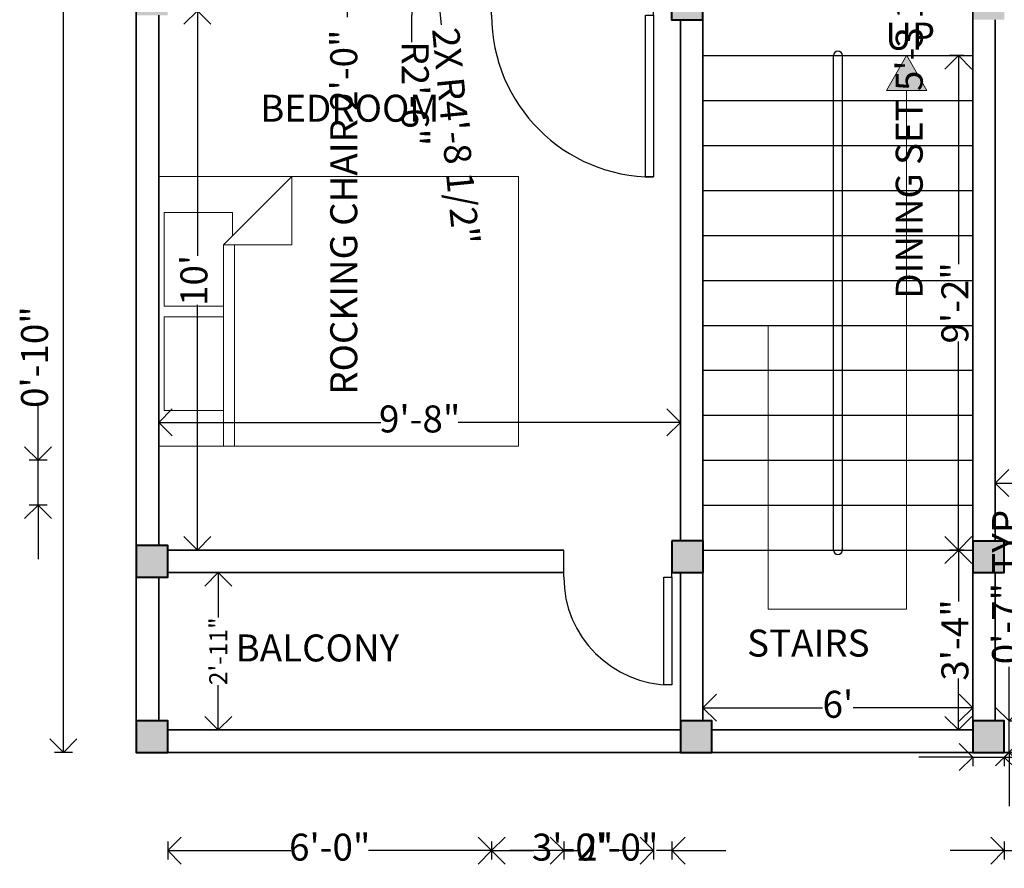
# Model space of a CAD drawing. Units: inches. Extents: x 261 to 714, y 97 to 573.
# Tile 1 of 5: x 322 to 541, y 97 to 286. Entities that reach past the tile are written whole.
import ezdxf

# ---------------------------------------------------------------- set-up
doc = ezdxf.new("R2010")
doc.units = ezdxf.units.IN
for name, color, linetype, lineweight in [('A-ANNO-DIMS', 2, 'Continuous', 18), ('A-ANNO-PATT', 1, 'Continuous', 13), ('A-ANNO-SYMB', 1, 'Continuous', 18), ('A-ANNO-TEXT', 7, 'Continuous', 18), ('A-AREA-IDEN', 7, 'Continuous', 25), ('A-COLS', 182, 'Continuous', 40), ('A-COLS-PATT', 172, 'Continuous', 13), ('A-DOOR', 182, 'Continuous', 25), ('A-FLOR-STRS', 182, 'Continuous', 25), ('A-FURN', 8, 'Continuous', 18), ('A-WALL', 182, 'Continuous', 35)]:
    doc.layers.add(name, color=color, linetype=linetype, lineweight=lineweight)
doc.styles.get("Standard").update_dxf_attribs({"font": 'arial.ttf'})
doc.dimstyles.new('ISO-25', dxfattribs={"dimtxt": 6, "dimasz": 6, "dimexe": 2, "dimexo": 2, "dimtad": 0, "dimdec": 1, "dimlunit": 3, "dimtxsty": 'Standard', "dimblk": 'OPEN90', "dimcen": 2.5, "dimclrd": 1, "dimclre": 1, "dimclrt": 1, "dimadec": 0, "dimazin": 0, "dimtfac": 1, "dimtdec": 1, "dimtmove": 0, "dimatfit": 3, "dimfxl": 2, "dimfxlon": 1, "dimarcsym": 0})

# ---------------------------------------------------------------- blocks, each defined once
blk = doc.blocks.new('*U4')
for p, q in [((0, 0), (0, -6)), ((36, 0), (36, -6))]:
    blk.add_line(p, q)
blk.add_lwpolyline([(0, 0), (0, 36), (1.75, 36), (1.75, 0)], close=True)
blk.add_arc((0, 0), 36, 0, 90)
blk = doc.blocks.new('*U6')
for p, q in [((0, 0), (0, -6)), ((24, 0), (24, -6))]:
    blk.add_line(p, q)
blk.add_lwpolyline([(0, 0), (0, 24), (1.75, 24), (1.75, 0)], close=True)
blk.add_arc((0, 0), 24, 0, 90)
blk = doc.blocks.new('_Open90')
at = {"color": 0, "linetype": 'ByBlock', "lineweight": -2}
for p, q in [((-0.5, 0.5), (0, 0)), ((0, 0), (-1, 0)), ((0, 0), (-0.5, -0.5))]:
    blk.add_line(p, q, dxfattribs=at)
blk = doc.blocks.new('*D19')
at = {"layer": 'A-ANNO-DIMS', "color": 0, "lineweight": -2, "transparency": 16777216}
for p, q in [((352.9, 194.06), (352.9, 198.06)), ((468.9, 194.06), (468.9, 198.06)), ((358.9, 196.06), (402.3, 196.06)), ((462.9, 196.06), (419.5, 196.06))]:
    blk.add_line(p, q, dxfattribs=at)
at = {"layer": 'Defpoints', "color": 0, "transparency": 16777216}
for p in [(468.9, 196.06), (352.9, 182.09), (468.9, 182.09)]:
    blk.add_point(p, dxfattribs=at)
at = {"layer": 'A-ANNO-DIMS', "color": 0, "lineweight": -2, "transparency": 16777216, "xscale": 6, "yscale": 6, "zscale": 6, "rotation": 180}
blk.add_blockref('_Open90', (352.9, 196.06), dxfattribs=at)
at = {"layer": 'A-ANNO-DIMS', "color": 0, "lineweight": -2, "transparency": 16777216, "xscale": 6, "yscale": 6, "zscale": 6}
blk.add_blockref('_Open90', (468.9, 196.06), dxfattribs=at)
at = {"layer": 'A-ANNO-DIMS', "color": 0, "transparency": 16777216, "insert": (410.9, 196.06), "char_height": 6, "attachment_point": 5}
blk.add_mtext('9\'-8"', dxfattribs=at)
blk = doc.blocks.new('*D20')
at = {"layer": 'A-ANNO-DIMS', "color": 0, "lineweight": -2, "transparency": 16777216}
for p, q in [((363.48, 287.66), (359.48, 287.66)), ((361.48, 281.66), (361.48, 233.09)), ((361.48, 173.66), (361.48, 222.22)), ((363.48, 167.66), (359.48, 167.66))]:
    blk.add_line(p, q, dxfattribs=at)
at = {"layer": 'Defpoints', "color": 0, "transparency": 16777216}
for p in [(378.83, 287.66), (361.48, 167.66), (378.83, 167.66)]:
    blk.add_point(p, dxfattribs=at)
at = {"layer": 'A-ANNO-DIMS', "color": 0, "lineweight": -2, "transparency": 16777216, "xscale": 6, "yscale": 6, "zscale": 6}
for p, rotation in [((361.48, 287.66), 90), ((361.48, 167.66), 270)]:
    blk.add_blockref('_Open90', p, dxfattribs=dict(at, rotation=rotation))
at = {"layer": 'A-ANNO-DIMS', "color": 0, "transparency": 16777216, "insert": (361.48, 227.66), "char_height": 6, "attachment_point": 5, "rotation": 90}
blk.add_mtext("10'", dxfattribs=at)
blk = doc.blocks.new('*D22')
at = {"layer": 'A-ANNO-DIMS', "color": 0, "lineweight": -2, "transparency": 16777216}
for p, q in [((538.9, 184.57), (538.9, 180.57)), ((654.9, 184.57), (654.9, 180.57)), ((544.9, 182.57), (588.3, 182.57)), ((648.9, 182.57), (605.5, 182.57))]:
    blk.add_line(p, q, dxfattribs=at)
at = {"layer": 'Defpoints', "color": 0, "transparency": 16777216}
for p in [(538.9, 189.8), (654.9, 189.8), (654.9, 182.57)]:
    blk.add_point(p, dxfattribs=at)
at = {"layer": 'A-ANNO-DIMS', "color": 0, "lineweight": -2, "transparency": 16777216, "xscale": 6, "yscale": 6, "zscale": 6, "rotation": 180}
blk.add_blockref('_Open90', (538.9, 182.57), dxfattribs=at)
at = {"layer": 'A-ANNO-DIMS', "color": 0, "lineweight": -2, "transparency": 16777216, "xscale": 6, "yscale": 6, "zscale": 6}
blk.add_blockref('_Open90', (654.9, 182.57), dxfattribs=at)
at = {"layer": 'A-ANNO-DIMS', "color": 0, "transparency": 16777216, "insert": (596.9, 182.57), "char_height": 6, "attachment_point": 5}
blk.add_mtext('9\'-8"', dxfattribs=at)
blk = doc.blocks.new('*D23')
at = {"layer": 'A-ANNO-DIMS', "color": 0, "lineweight": -2, "transparency": 16777216}
for p, q in [((368.12, 162.66), (364.12, 162.66)), ((366.12, 156.66), (366.12, 152.69)), ((366.12, 133.66), (366.12, 137.63)), ((368.12, 127.66), (364.12, 127.66))]:
    blk.add_line(p, q, dxfattribs=at)
at = {"layer": 'Defpoints', "color": 0, "transparency": 16777216}
for p in [(380.54, 162.66), (366.12, 127.66), (380.54, 127.66)]:
    blk.add_point(p, dxfattribs=at)
at = {"layer": 'A-ANNO-DIMS', "color": 0, "lineweight": -2, "transparency": 16777216, "xscale": 6, "yscale": 6, "zscale": 6}
for p, rotation in [((366.12, 162.66), 90), ((366.12, 127.66), 270)]:
    blk.add_blockref('_Open90', p, dxfattribs=dict(at, rotation=rotation))
at = {"layer": 'A-ANNO-DIMS', "color": 0, "transparency": 16777216, "insert": (366.12, 145.16), "char_height": 6, "attachment_point": 5, "rotation": 90}
blk.add_mtext('{\\H0.66667x;2\'-11"}', dxfattribs=at)
blk = doc.blocks.new('*D25')
at = {"layer": 'A-ANNO-DIMS', "color": 0, "lineweight": -2, "transparency": 16777216}
for p, q in [((473.9, 134.58), (473.9, 130.58)), ((533.9, 134.58), (533.9, 130.58)), ((479.9, 132.58), (500.5, 132.58)), ((527.9, 132.58), (507.31, 132.58))]:
    blk.add_line(p, q, dxfattribs=at)
at = {"layer": 'Defpoints', "color": 0, "transparency": 16777216}
for p in [(473.9, 138.97), (533.9, 138.97), (533.9, 132.58)]:
    blk.add_point(p, dxfattribs=at)
at = {"layer": 'A-ANNO-DIMS', "color": 0, "lineweight": -2, "transparency": 16777216, "xscale": 6, "yscale": 6, "zscale": 6, "rotation": 180}
blk.add_blockref('_Open90', (473.9, 132.58), dxfattribs=at)
at = {"layer": 'A-ANNO-DIMS', "color": 0, "lineweight": -2, "transparency": 16777216, "xscale": 6, "yscale": 6, "zscale": 6}
blk.add_blockref('_Open90', (533.9, 132.58), dxfattribs=at)
at = {"layer": 'A-ANNO-DIMS', "color": 0, "transparency": 16777216, "insert": (503.9, 132.58), "char_height": 6, "attachment_point": 5}
blk.add_mtext("6'", dxfattribs=at)
blk = doc.blocks.new('*D26')
at = {"layer": 'A-ANNO-DIMS', "color": 0, "lineweight": -2, "transparency": 16777216}
for p, q in [((531.9, 277.66), (528.69, 277.66)), ((530.69, 271.66), (530.69, 231.26)), ((530.69, 173.66), (530.69, 214.06)), ((531.9, 167.66), (528.69, 167.66))]:
    blk.add_line(p, q, dxfattribs=at)
at = {"layer": 'Defpoints', "color": 0, "transparency": 16777216}
for p in [(533.9, 277.66), (530.69, 167.66), (533.9, 167.66)]:
    blk.add_point(p, dxfattribs=at)
at = {"layer": 'A-ANNO-DIMS', "color": 0, "lineweight": -2, "transparency": 16777216, "xscale": 6, "yscale": 6, "zscale": 6}
for p, rotation in [((530.69, 277.66), 90), ((530.69, 167.66), 270)]:
    blk.add_blockref('_Open90', p, dxfattribs=dict(at, rotation=rotation))
at = {"layer": 'A-ANNO-DIMS', "color": 0, "transparency": 16777216, "insert": (530.69, 222.66), "char_height": 6, "attachment_point": 5, "rotation": 90}
blk.add_mtext('9\'-2"', dxfattribs=at)
blk = doc.blocks.new('*D27')
at = {"layer": 'A-ANNO-DIMS', "color": 0, "lineweight": -2, "transparency": 16777216}
for p, q in [((530.69, 167.66), (532.69, 167.66)), ((530.69, 161.66), (530.69, 156.25)), ((530.69, 133.66), (530.69, 139.06)), ((530.69, 127.66), (532.69, 127.66))]:
    blk.add_line(p, q, dxfattribs=at)
at = {"layer": 'Defpoints', "color": 0, "transparency": 16777216}
for p in [(530.69, 167.66), (530.69, 127.66), (530.69, 127.66)]:
    blk.add_point(p, dxfattribs=at)
at = {"layer": 'A-ANNO-DIMS', "color": 0, "lineweight": -2, "transparency": 16777216, "xscale": 6, "yscale": 6, "zscale": 6}
for p, rotation in [((530.69, 167.66), 90), ((530.69, 127.66), 270)]:
    blk.add_blockref('_Open90', p, dxfattribs=dict(at, rotation=rotation))
at = {"layer": 'A-ANNO-DIMS', "color": 0, "transparency": 16777216, "insert": (530.69, 147.66), "char_height": 6, "attachment_point": 5, "rotation": 90}
blk.add_mtext('3\'-4"', dxfattribs=at)
blk = doc.blocks.new('Bed - Queen')
for p, q in [((0, -80.00003), (0, 0)), ((0, 0), (59.99999, 0)), ((59.99999, 0), (59.99999, -80.00003)), ((7.99999, -1.2), (28.79998, -1.2)), ((7.99999, -14.4), (7.99999, -1.2)), ((28.79998, -1.2), (28.79998, -14.4)), ((31.19999, -1.2), (51.99999, -1.2)), ((31.19999, -14.4), (31.19999, -1.2)), ((51.99999, -1.2), (51.99999, -16.4)), ((0, -14.4), (44.8, -14.4)), ((59.99999, -29.6), (44.8, -14.4)), ((44.8, -14.4), (44.8, -29.6)), ((44.8, -16.8), (0, -16.8)), ((51.99999, -16.4), (46.79936, -16.4)), ((44.8, -29.6), (59.99999, -29.6)), ((59.99999, -80.00003), (0, -80.00003))]:
    blk.add_line(p, q)
blk = doc.blocks.new('*D36')
at = {"layer": 'A-ANNO-DIMS', "color": 0, "lineweight": -2, "transparency": 16777216}
for p, q in [((333.7, 542.66), (329.7, 542.66)), ((331.7, 536.66), (331.7, 338.37)), ((331.7, 128.66), (331.7, 326.94)), ((333.7, 122.66), (329.7, 122.66))]:
    blk.add_line(p, q, dxfattribs=at)
at = {"layer": 'Defpoints', "color": 0, "transparency": 16777216}
for p in [(347.9, 542.66), (331.7, 122.66), (347.9, 122.66)]:
    blk.add_point(p, dxfattribs=at)
at = {"layer": 'A-ANNO-DIMS', "color": 0, "lineweight": -2, "transparency": 16777216, "xscale": 6, "yscale": 6, "zscale": 6}
for p, rotation in [((331.7, 542.66), 90), ((331.7, 122.66), 270)]:
    blk.add_blockref('_Open90', p, dxfattribs=dict(at, rotation=rotation))
at = {"layer": 'A-ANNO-DIMS', "color": 0, "transparency": 16777216, "insert": (331.7, 332.66), "char_height": 6, "attachment_point": 5, "rotation": 90}
blk.add_mtext("35'", dxfattribs=at)
blk = doc.blocks.new('COLUMN-7IN-SQUARE')
blk.add_lwpolyline([(0, 7), (0, 2), (0, 0), (2, 0), (7, 0), (7, 2), (7, 7)], close=True)
blk = doc.blocks.new('*D41')
at = {"layer": 'A-ANNO-DIMS', "color": 1, "lineweight": -2, "transparency": 16777216}
for p, q in [((527.9, 121.61), (521.9, 121.61)), ((533.9, 121.61), (533.9, 119.61)), ((533.9, 121.61), (540.9, 121.61)), ((540.9, 121.61), (540.9, 119.61)), ((546.9, 121.61), (552.9, 121.61))]:
    blk.add_line(p, q, dxfattribs=at)
at = {"layer": 'Defpoints', "color": 0, "transparency": 16777216}
for p in [(533.9, 122.66), (540.9, 122.66), (540.9, 121.61)]:
    blk.add_point(p, dxfattribs=at)
at = {"layer": 'A-ANNO-DIMS', "color": 1, "lineweight": -2, "transparency": 16777216, "xscale": 6, "yscale": 6, "zscale": 6}
blk.add_blockref('_Open90', (533.9, 121.61), dxfattribs=at)
at = {"layer": 'A-ANNO-DIMS', "color": 1, "lineweight": -2, "transparency": 16777216, "xscale": 6, "yscale": 6, "zscale": 6, "rotation": 180}
blk.add_blockref('_Open90', (540.9, 121.61), dxfattribs=at)
at = {"layer": 'A-ANNO-DIMS', "color": 1, "transparency": 16777216, "insert": (591.11, 121.61), "char_height": 6, "attachment_point": 5}
blk.add_mtext('COLUMN 0\'-7" TYP.', dxfattribs=at)
blk = doc.blocks.new('*D42')
at = {"layer": 'A-ANNO-DIMS', "color": 1, "lineweight": -2, "transparency": 16777216}
for p, q in [((541.95, 135.66), (541.95, 141.66)), ((541.95, 129.66), (543.95, 129.66)), ((541.95, 122.66), (541.95, 129.66)), ((541.95, 122.66), (543.95, 122.66)), ((541.95, 116.66), (541.95, 110.66))]:
    blk.add_line(p, q, dxfattribs=at)
at = {"layer": 'Defpoints', "color": 0, "transparency": 16777216}
for p in [(540.9, 129.66), (541.95, 129.66), (540.9, 122.66)]:
    blk.add_point(p, dxfattribs=at)
at = {"layer": 'A-ANNO-DIMS', "color": 1, "lineweight": -2, "transparency": 16777216, "xscale": 6, "yscale": 6, "zscale": 6}
for p, rotation in [((541.95, 129.66), 270), ((541.95, 122.66), 90)]:
    blk.add_blockref('_Open90', p, dxfattribs=dict(at, rotation=rotation))
at = {"layer": 'A-ANNO-DIMS', "color": 1, "transparency": 16777216, "insert": (541.95, 160.57), "char_height": 6, "attachment_point": 5, "rotation": 90}
blk.add_mtext('0\'-7" TYP.', dxfattribs=at)
blk = doc.blocks.new('*D51')
at = {"layer": 'A-ANNO-DIMS', "color": 1, "lineweight": -2, "transparency": 16777216}
for p, q in [((522.54, 372.81), (518.54, 372.81)), ((520.54, 366.81), (520.54, 315.39)), ((522.54, 309.39), (518.54, 309.39)), ((520.54, 309.39), (520.54, 303.39))]:
    blk.add_line(p, q, dxfattribs=at)
at = {"layer": 'Defpoints', "color": 0, "transparency": 16777216}
for p in [(530.06, 372.81), (520.54, 309.39), (530.06, 309.39)]:
    blk.add_point(p, dxfattribs=at)
at = {"layer": 'A-ANNO-DIMS', "color": 1, "lineweight": -2, "transparency": 16777216, "xscale": 6, "yscale": 6, "zscale": 6}
for p, rotation in [((520.54, 372.81), 90), ((520.54, 309.39), 270)]:
    blk.add_blockref('_Open90', p, dxfattribs=dict(at, rotation=rotation))
at = {"layer": 'A-ANNO-DIMS', "color": 1, "transparency": 16777216, "insert": (520.54, 262.8), "char_height": 6, "attachment_point": 5, "rotation": 90}
blk.add_mtext('DINING SET 5\'-3 1/2"', dxfattribs=at)
blk = doc.blocks.new('*D53')
at = {"layer": 'A-ANNO-DIMS', "color": 1, "lineweight": -2, "transparency": 16777216}
for p, q in [((396.37, 316.03), (392.8, 316.03)), ((394.8, 310.03), (394.8, 298.22)), ((396.37, 292.22), (392.8, 292.22)), ((394.8, 292.22), (394.8, 286.22))]:
    blk.add_line(p, q, dxfattribs=at)
at = {"layer": 'Defpoints', "color": 0, "transparency": 16777216}
for p in [(398.37, 316.03), (394.8, 292.22), (398.37, 292.22)]:
    blk.add_point(p, dxfattribs=at)
at = {"layer": 'A-ANNO-DIMS', "color": 1, "lineweight": -2, "transparency": 16777216, "xscale": 6, "yscale": 6, "zscale": 6}
for p, rotation in [((394.8, 316.03), 90), ((394.8, 292.22), 270)]:
    blk.add_blockref('_Open90', p, dxfattribs=dict(at, rotation=rotation))
at = {"layer": 'A-ANNO-DIMS', "color": 1, "transparency": 16777216, "insert": (394.8, 242.84), "char_height": 6, "attachment_point": 5, "rotation": 90}
blk.add_mtext('ROCKING CHAIR 2\'-0"', dxfattribs=at)
blk = doc.blocks.new('*D61')
at = {"layer": 'A-ANNO-DIMS', "color": 1, "lineweight": -2, "transparency": 16777216}
for p, q in [((354.9, 102.81), (354.9, 98.81)), ((360.9, 100.81), (382.29, 100.81)), ((420.9, 100.81), (399.52, 100.81)), ((426.9, 102.81), (426.9, 98.81))]:
    blk.add_line(p, q, dxfattribs=at)
at = {"layer": 'Defpoints', "color": 0, "transparency": 16777216}
for p in [(354.9, 287.66), (426.9, 287.66), (426.9, 100.81)]:
    blk.add_point(p, dxfattribs=at)
at = {"layer": 'A-ANNO-DIMS', "color": 1, "lineweight": -2, "transparency": 16777216, "xscale": 6, "yscale": 6, "zscale": 6, "rotation": 180}
blk.add_blockref('_Open90', (354.9, 100.81), dxfattribs=at)
at = {"layer": 'A-ANNO-DIMS', "color": 1, "lineweight": -2, "transparency": 16777216, "xscale": 6, "yscale": 6, "zscale": 6}
blk.add_blockref('_Open90', (426.9, 100.81), dxfattribs=at)
at = {"layer": 'A-ANNO-DIMS', "color": 1, "transparency": 16777216, "insert": (390.9, 100.81), "char_height": 6, "attachment_point": 5}
blk.add_mtext('6\'-0"', dxfattribs=at)
blk = doc.blocks.new('*D62')
at = {"layer": 'A-ANNO-DIMS', "color": 1, "lineweight": -2, "transparency": 16777216}
for p, q in [((426.9, 102.81), (426.9, 98.81)), ((432.9, 100.81), (436.31, 100.81)), ((456.9, 100.81), (453.5, 100.81)), ((462.9, 102.81), (462.9, 98.81))]:
    blk.add_line(p, q, dxfattribs=at)
at = {"layer": 'Defpoints', "color": 0, "transparency": 16777216}
for p in [(426.9, 287.66), (462.9, 287.66), (462.9, 100.81)]:
    blk.add_point(p, dxfattribs=at)
at = {"layer": 'A-ANNO-DIMS', "color": 1, "lineweight": -2, "transparency": 16777216, "xscale": 6, "yscale": 6, "zscale": 6, "rotation": 180}
blk.add_blockref('_Open90', (426.9, 100.81), dxfattribs=at)
at = {"layer": 'A-ANNO-DIMS', "color": 1, "lineweight": -2, "transparency": 16777216, "xscale": 6, "yscale": 6, "zscale": 6}
blk.add_blockref('_Open90', (462.9, 100.81), dxfattribs=at)
at = {"layer": 'A-ANNO-DIMS', "color": 1, "transparency": 16777216, "insert": (444.9, 100.81), "char_height": 6, "attachment_point": 5}
blk.add_mtext('3\'-0"', dxfattribs=at)
blk = doc.blocks.new('*D65')
at = {"layer": 'A-ANNO-DIMS', "color": 1, "lineweight": -2, "transparency": 16777216}
for p, q in [((436.95, 100.81), (430.95, 100.81)), ((442.95, 102.81), (442.95, 98.81)), ((442.95, 100.81), (446.29, 100.81)), ((466.95, 100.81), (463.6, 100.81)), ((466.95, 102.81), (466.95, 98.81)), ((472.95, 100.81), (478.95, 100.81))]:
    blk.add_line(p, q, dxfattribs=at)
at = {"layer": 'Defpoints', "color": 0, "transparency": 16777216}
for p in [(442.95, 162.66), (466.95, 162.69), (466.95, 100.81)]:
    blk.add_point(p, dxfattribs=at)
at = {"layer": 'A-ANNO-DIMS', "color": 1, "lineweight": -2, "transparency": 16777216, "xscale": 6, "yscale": 6, "zscale": 6}
blk.add_blockref('_Open90', (442.95, 100.81), dxfattribs=at)
at = {"layer": 'A-ANNO-DIMS', "color": 1, "lineweight": -2, "transparency": 16777216, "xscale": 6, "yscale": 6, "zscale": 6, "rotation": 180}
blk.add_blockref('_Open90', (466.95, 100.81), dxfattribs=at)
at = {"layer": 'A-ANNO-DIMS', "color": 1, "transparency": 16777216, "insert": (454.95, 100.81), "char_height": 6, "attachment_point": 5}
blk.add_mtext('2\'-0"', dxfattribs=at)
blk = doc.blocks.new('*D66')
at = {"layer": 'A-ANNO-DIMS', "color": 1, "lineweight": -2, "transparency": 16777216}
for p, q in [((534.9, 100.81), (528.9, 100.81)), ((540.9, 102.81), (540.9, 98.81)), ((540.9, 100.81), (544.25, 100.81)), ((564.9, 100.81), (561.55, 100.81)), ((564.9, 102.81), (564.9, 98.81)), ((570.9, 100.81), (576.9, 100.81))]:
    blk.add_line(p, q, dxfattribs=at)
at = {"layer": 'Defpoints', "color": 0, "transparency": 16777216}
for p in [(540.9, 162.66), (564.9, 162.66), (564.9, 100.81)]:
    blk.add_point(p, dxfattribs=at)
at = {"layer": 'A-ANNO-DIMS', "color": 1, "lineweight": -2, "transparency": 16777216, "xscale": 6, "yscale": 6, "zscale": 6}
blk.add_blockref('_Open90', (540.9, 100.81), dxfattribs=at)
at = {"layer": 'A-ANNO-DIMS', "color": 1, "lineweight": -2, "transparency": 16777216, "xscale": 6, "yscale": 6, "zscale": 6, "rotation": 180}
blk.add_blockref('_Open90', (564.9, 100.81), dxfattribs=at)
at = {"layer": 'A-ANNO-DIMS', "color": 1, "transparency": 16777216, "insert": (552.9, 100.81), "char_height": 6, "attachment_point": 5}
blk.add_mtext('2\'-0"', dxfattribs=at)
blk = doc.blocks.new('*D67')
at = {"layer": 'A-ANNO-DIMS', "color": 1, "lineweight": -2, "transparency": 16777216}
for p, q in [((326.05, 193.66), (326.05, 199.66)), ((328.05, 187.66), (324.05, 187.66)), ((326.05, 177.66), (326.05, 187.66)), ((328.05, 177.66), (324.05, 177.66)), ((326.05, 171.66), (326.05, 165.66))]:
    blk.add_line(p, q, dxfattribs=at)
at = {"layer": 'Defpoints', "color": 0, "transparency": 16777216}
for p in [(326.05, 187.66), (473.9, 187.66), (473.9, 177.66)]:
    blk.add_point(p, dxfattribs=at)
at = {"layer": 'A-ANNO-DIMS', "color": 1, "lineweight": -2, "transparency": 16777216, "xscale": 6, "yscale": 6, "zscale": 6}
for p, rotation in [((326.05, 187.66), 270), ((326.05, 177.66), 90)]:
    blk.add_blockref('_Open90', p, dxfattribs=dict(at, rotation=rotation))
at = {"layer": 'A-ANNO-DIMS', "color": 1, "transparency": 16777216, "insert": (326.05, 210.59), "char_height": 6, "attachment_point": 5, "rotation": 90}
blk.add_mtext('0\'-10"', dxfattribs=at)
blk = doc.blocks.new('*D81')
at = {"layer": 'A-ANNO-DIMS', "color": 1, "lineweight": -2, "transparency": 16777216}
for p, q in [((409.15, 352.86), (414.62, 296.45)), ((415.78, 284.51), (415.2, 290.48))]:
    blk.add_line(p, q, dxfattribs=at)
at = {"layer": 'Defpoints', "color": 0, "transparency": 16777216}
for p in [(409.15, 352.86), (414.62, 296.45)]:
    blk.add_point(p, dxfattribs=at)
at = {"layer": 'A-ANNO-DIMS', "color": 1, "lineweight": -2, "transparency": 16777216, "xscale": 6, "yscale": 6, "zscale": 6, "rotation": 95.53759783759804}
blk.add_blockref('_Open90', (414.62, 296.45), dxfattribs=at)
at = {"layer": 'A-ANNO-DIMS', "color": 1, "transparency": 16777216, "insert": (418.19, 259.66), "char_height": 6, "attachment_point": 5, "rotation": 275.5376}
blk.add_mtext('2X R4\'-8 1/2"', dxfattribs=at)
blk = doc.blocks.new('*D82')
at = {"layer": 'A-ANNO-DIMS', "color": 1, "lineweight": -2, "transparency": 16777216}
for p, q in [((409.15, 322.72), (409.15, 292.66)), ((409.15, 280.66), (409.15, 286.66))]:
    blk.add_line(p, q, dxfattribs=at)
at = {"layer": 'Defpoints', "color": 0, "transparency": 16777216}
for p in [(409.15, 322.72), (409.15, 292.66)]:
    blk.add_point(p, dxfattribs=at)
at = {"layer": 'A-ANNO-DIMS', "color": 1, "lineweight": -2, "transparency": 16777216, "xscale": 6, "yscale": 6, "zscale": 6, "rotation": 90.00021153640085}
blk.add_blockref('_Open90', (409.15, 292.66), dxfattribs=at)
at = {"layer": 'A-ANNO-DIMS', "color": 1, "transparency": 16777216, "insert": (409.15, 269.19), "char_height": 6, "attachment_point": 5, "rotation": 270.0002}
blk.add_mtext('R2\'-6"', dxfattribs=at)

msp = doc.modelspace()

# ---------------------------------------------------------------- hatches: boundary and pattern name
at = {"layer": 'A-ANNO-PATT'}
h = msp.add_hatch(color=256, dxfattribs=at)
h.dxf.hatch_style = 1
h.paths.add_polyline_path([(519.22, 277.66), (519.19, 277.66), (514.71, 269.89), (523.71, 269.89)])
at = {"layer": 'A-COLS-PATT'}
h = msp.add_hatch(color=256, dxfattribs=at)
h.dxf.hatch_style = 1
h.paths.add_polyline_path([(354.9, 542.66), (347.9, 542.66), (347.9, 535.66), (354.9, 535.66)])
h.paths.add_polyline_path([(539.9, 542.66), (532.9, 542.66), (532.9, 537.66), (532.9, 535.66), (534.9, 535.66), (539.9, 535.66), (539.9, 537.66)])
h.paths.add_polyline_path([(474.9, 542.66), (467.9, 542.66), (467.9, 537.66), (467.9, 535.66), (469.9, 535.66), (474.9, 535.66), (474.9, 537.66)])
h.paths.add_polyline_path([(659.9, 542.66), (652.9, 542.66), (652.9, 537.66), (652.9, 535.66), (654.9, 535.66), (659.9, 535.66)])
h.paths.add_polyline_path([(659.9, 395.66), (652.88, 395.66), (652.88, 390.66), (652.88, 388.66), (654.88, 388.66), (659.9, 388.66)])
h.paths.add_polyline_path([(539.9, 395.66), (532.9, 395.66), (532.9, 390.66), (532.9, 388.66), (534.9, 388.66), (539.9, 388.66), (539.9, 390.66)])
h.paths.add_polyline_path([(473.9, 395.66), (466.9, 395.66), (466.9, 394.66), (466.9, 388.66), (473.9, 388.66)])
h.paths.add_polyline_path([(354.9, 394.66), (347.9, 394.66), (347.9, 389.66), (347.9, 387.66), (349.9, 387.66), (354.9, 387.66), (354.9, 389.66)])
h.paths.add_polyline_path([(540.9, 292.66), (533.9, 292.66), (533.9, 287.66), (533.9, 285.66), (535.9, 285.66), (540.9, 285.66), (540.9, 287.66)])
h.paths.add_polyline_path([(659.9, 294.66), (652.88, 294.66), (652.88, 289.66), (652.88, 287.66), (654.88, 287.66), (659.9, 287.66)])
h.paths.add_polyline_path([(473.9, 292.66), (466.9, 292.66), (466.9, 287.66), (466.9, 285.66), (468.9, 285.66), (473.9, 285.66), (473.9, 287.66)])
h.paths.add_polyline_path([(354.9, 293.66), (347.9, 293.66), (347.9, 288.66), (347.9, 286.66), (349.9, 286.66), (354.9, 286.66), (354.9, 288.66)])
h.paths.add_polyline_path([(354.9, 129.66), (347.9, 129.66), (347.9, 124.66), (347.9, 122.66), (349.9, 122.66), (354.9, 122.66), (354.9, 124.66)])
h.paths.add_polyline_path([(354.9, 168.66), (347.9, 168.66), (347.9, 163.66), (347.9, 161.66), (349.9, 161.66), (354.9, 161.66), (354.9, 163.66)])
h.paths.add_polyline_path([(473.9, 169.69), (466.95, 169.69), (466.95, 164.69), (466.95, 162.69), (468.95, 162.69), (473.9, 162.69)])
h.paths.add_polyline_path([(475.9, 129.66), (468.9, 129.66), (468.9, 124.66), (468.9, 122.66), (470.9, 122.66), (475.9, 122.66), (475.9, 124.66)])
h.paths.add_polyline_path([(540.9, 129.66), (533.9, 129.66), (533.9, 124.66), (533.9, 122.66), (535.9, 122.66), (540.9, 122.66), (540.9, 124.66)])
h.paths.add_polyline_path([(540.9, 169.66), (533.9, 169.66), (533.9, 164.66), (533.9, 162.66), (535.9, 162.66), (540.9, 162.66), (540.9, 164.66)])
h.paths.add_polyline_path([(659.9, 169.66), (652.9, 169.66), (652.9, 164.66), (652.9, 162.66), (654.9, 162.66), (659.9, 162.66)])
h.paths.add_polyline_path([(659.9, 129.66), (652.9, 129.66), (652.9, 124.66), (652.9, 122.66), (654.9, 122.66), (659.9, 122.66)])

# ---------------------------------------------------------------- linework, layer by layer
at = {"layer": 'A-ANNO-SYMB'}
for p, q in [((519.19, 277.66), (514.71, 269.89)), ((523.71, 269.89), (519.22, 277.66)), ((514.71, 269.89), (523.71, 269.89)), ((519.19, 154.49), (519.19, 269.89)), ((488.4, 217.66), (488.4, 154.49)), ((488.4, 154.49), (519.19, 154.49))]:
    msp.add_line(p, q, dxfattribs=at)
at = {"layer": 'A-FLOR-STRS'}
for p, q in [((473.9, 277.66), (533.9, 277.66)), ((502.9, 167.66), (502.9, 277.66)), ((504.9, 167.66), (504.9, 277.66)), ((473.9, 267.66), (533.9, 267.66)), ((473.9, 257.66), (533.9, 257.66)), ((473.9, 247.66), (533.9, 247.66)), ((473.9, 237.66), (533.9, 237.66)), ((473.9, 227.66), (533.9, 227.66)), ((473.9, 217.66), (533.9, 217.66)), ((473.9, 207.66), (533.9, 207.66)), ((473.9, 197.66), (533.9, 197.66)), ((473.9, 187.66), (533.9, 187.66)), ((473.9, 177.66), (533.9, 177.66)), ((473.9, 167.66), (533.9, 167.66))]:
    msp.add_line(p, q, dxfattribs=at)
for centre, start, end in [((503.9, 277.66), 0, 180), ((503.9, 167.66), 180, 0)]:
    msp.add_arc(centre, 1, start, end, dxfattribs=at)
at = {"layer": 'A-WALL'}
for p, q in [((347.9, 542.66), (347.9, 122.66)), ((473.9, 292.66), (473.9, 129.66)), ((533.9, 292.66), (533.9, 127.66)), ((352.9, 286.66), (352.9, 168.66)), ((468.9, 285.66), (468.9, 169.69)), ((538.9, 285.66), (538.9, 169.66)), ((354.9, 167.66), (442.95, 167.66)), ((354.9, 162.66), (442.95, 162.66)), ((468.9, 162.69), (468.9, 129.66)), ((468.9, 162.66), (473.9, 162.66)), ((533.9, 162.66), (538.9, 162.66)), ((538.9, 162.66), (538.9, 129.66)), ((352.9, 161.66), (352.9, 129.66)), ((354.9, 127.66), (468.9, 127.66)), ((475.9, 127.66), (533.9, 127.66)), ((347.9, 122.66), (659.9, 122.66))]:
    msp.add_line(p, q, dxfattribs=at)

# ---------------------------------------------------------------- block references
at = {"layer": 'A-COLS'}
for p in [(466.9, 285.66), (347.9, 161.66), (466.95, 162.69), (533.9, 162.66), (347.9, 122.66), (468.9, 122.66), (533.9, 122.66)]:
    msp.add_blockref('COLUMN-7IN-SQUARE', p, dxfattribs=at)
at = {"layer": 'A-DOOR', "rotation": 180}
for name, p in [('*U4', (462.9, 286.66)), ('*U6', (466.95, 161.66))]:
    msp.add_blockref(name, p, dxfattribs=at)
at = {"layer": 'A-FURN', "rotation": 90}
msp.add_blockref('Bed - Queen', (352.9, 190.75), dxfattribs=at)

# ---------------------------------------------------------------- texts
at = {"layer": 'A-ANNO-TEXT', "insert": (514.43, 285), "char_height": 6, "attachment_point": 1}
msp.add_mtext_dynamic_manual_height_columns('{UP}', width=11.3241, gutter_width=12.5, heights=[0], dxfattribs=at)
at = {"layer": 'A-AREA-IDEN', "char_height": 6, "attachment_point": 1}
for s, insert in [('{BEDROOM}', (375.43, 268.96)), ('{BALCONY}', (369.97, 148.89)), ('{STAIRS}', (483.71, 149.97))]:
    msp.add_mtext_dynamic_manual_height_columns(s, width=60.8654, gutter_width=12.5, heights=[0], dxfattribs=dict(at, insert=insert))

# ---------------------------------------------------------------- dimensions: what is measured, and where the dimension line sits
at = {"layer": 'A-ANNO-DIMS'}
for base, p1, p2, override, picture, middle in [((331.7, 122.66), (347.9, 542.66), (347.9, 122.66), {"dimclrd": 0, "dimclre": 0, "dimclrt": 0}, '*D36', (331.7, 332.66)), ((361.48, 167.66), (378.83, 287.66), (378.83, 167.66), {"dimclrd": 0, "dimclre": 0, "dimclrt": 0}, '*D20', (361.48, 227.66)), ((326.05, 187.66), (473.9, 177.66), (473.9, 187.66), {"dimdec": 1, "dimlfac": 1, "dimrnd": 0, "dimzin": 1, "dimdsep": 46, "dimlunit": 4, "dimfrac": 2}, '*D67', (326.05, 210.59)), ((530.69, 127.66), (530.69, 167.66), (530.69, 127.66), {"dimclrd": 0, "dimclre": 0, "dimclrt": 0}, '*D27', (530.69, 147.66))]:
    dim = msp.add_linear_dim(base=base, p1=p1, p2=p2, angle=90, dimstyle='ISO-25', override=override, dxfattribs=at)
    dim.commit()
    dim.dimension.update_dxf_attribs({"geometry": picture, "text_midpoint": middle})
for base, p1, p2, angle, text, override, picture, middle in [((520.54, 309.39), (530.06, 372.81), (530.06, 309.39), 270, 'DINING SET <>', {"dimdec": 1, "dimlfac": 1, "dimrnd": 0, "dimzin": 1, "dimdsep": 46, "dimlunit": 4, "dimfrac": 2}, '*D51', (520.54, 262.8)), ((394.8, 292.22), (398.37, 316.03), (398.37, 292.22), 270, 'ROCKING CHAIR <>', {"dimdec": 1, "dimlfac": 1, "dimrnd": 0, "dimzin": 1, "dimdsep": 46, "dimlunit": 4, "dimfrac": 2}, '*D53', (394.8, 242.84)), ((541.95, 129.66), (540.9, 122.66), (540.9, 129.66), 90, '<> TYP.', {"dimdec": 1, "dimlfac": 1, "dimrnd": 0, "dimzin": 1, "dimdsep": 46, "dimlunit": 4, "dimfrac": 2}, '*D42', (541.95, 160.57)), ((366.12, 127.66), (380.54, 162.66), (380.54, 127.66), 90, '{\\H0.66667x;<>}', {"dimclrd": 0, "dimclre": 0, "dimclrt": 0}, '*D23', (366.12, 145.16))]:
    dim = msp.add_linear_dim(base=base, p1=p1, p2=p2, angle=angle, text=text, dimstyle='ISO-25', override=override, dxfattribs=at)
    dim.commit()
    dim.dimension.update_dxf_attribs({"geometry": picture, "text_midpoint": middle})
dim = msp.add_radius_dim(center=(409.15, 352.86), mpoint=(414.62, 296.45), text='2X <>', dimstyle='ISO-25', override={"dimdec": 1, "dimlfac": 1, "dimrnd": 0, "dimzin": 1, "dimdsep": 46, "dimlunit": 4, "dimfrac": 2}, dxfattribs=at)
dim.commit()
dim.dimension.update_dxf_attribs({"geometry": '*D81', "text_midpoint": (418.19, 259.66)})
dim = msp.add_radius_dim(center=(409.15, 322.72), mpoint=(409.15, 292.66), dimstyle='ISO-25', override={"dimdec": 1, "dimlfac": 1, "dimrnd": 0, "dimzin": 1, "dimdsep": 46, "dimlunit": 4, "dimfrac": 2}, dxfattribs=at)
dim.commit()
dim.dimension.update_dxf_attribs({"geometry": '*D82', "text_midpoint": (409.15, 269.19)})
for base, p1, p2, override, picture, middle in [((426.9, 100.81), (354.9, 287.66), (426.9, 287.66), {"dimdec": 1, "dimlfac": 1, "dimrnd": 0, "dimzin": 1, "dimdsep": 46, "dimlunit": 4, "dimfrac": 2}, '*D61', (390.9, 100.81)), ((462.9, 100.81), (426.9, 287.66), (462.9, 287.66), {"dimdec": 1, "dimlfac": 1, "dimrnd": 0, "dimzin": 1, "dimdsep": 46, "dimlunit": 4, "dimfrac": 2}, '*D62', (444.9, 100.81)), ((468.9, 196.06), (352.9, 182.09), (468.9, 182.09), {"dimclrd": 0, "dimclre": 0, "dimclrt": 0}, '*D19', (410.9, 196.06)), ((466.95, 100.81), (442.95, 162.66), (466.95, 162.69), {"dimdec": 1, "dimlfac": 1, "dimrnd": 0, "dimzin": 1, "dimdsep": 46, "dimlunit": 4, "dimfrac": 2}, '*D65', (454.95, 100.81)), ((564.9, 100.81), (540.9, 162.66), (564.9, 162.66), {"dimdec": 1, "dimlfac": 1, "dimrnd": 0, "dimzin": 1, "dimdsep": 46, "dimlunit": 4, "dimfrac": 2}, '*D66', (552.9, 100.81))]:
    dim = msp.add_linear_dim(base=base, p1=p1, p2=p2, dimstyle='ISO-25', override=override, dxfattribs=at)
    dim.commit()
    dim.dimension.update_dxf_attribs({"geometry": picture, "text_midpoint": middle})
dim = msp.add_linear_dim(base=(530.69, 167.66), p1=(533.9, 277.66), p2=(533.9, 167.66), angle=90, dimstyle='ISO-25', override={"dimclrd": 0, "dimclre": 0, "dimclrt": 0}, dxfattribs=at)
dim.commit()
dim.dimension.update_dxf_attribs({"geometry": '*D26', "text_midpoint": (530.69, 222.66), "dimtype": 160})
dim = msp.add_linear_dim(base=(654.9, 182.57), p1=(538.9, 189.8), p2=(654.9, 189.8), dimstyle='ISO-25', override={"dimclrd": 0, "dimclre": 0, "dimclrt": 0}, dxfattribs=at)
dim.commit()
dim.dimension.update_dxf_attribs({"geometry": '*D22', "text_midpoint": (596.9, 182.57), "dimtype": 160})
for base, p1, p2, text, override, picture, middle in [((533.9, 132.58), (473.9, 138.97), (533.9, 138.97), "6'", {"dimclrd": 0, "dimclre": 0, "dimclrt": 0}, '*D25', (503.9, 132.58)), ((540.9, 121.61), (533.9, 122.66), (540.9, 122.66), 'COLUMN <> TYP.', {"dimdec": 1, "dimlfac": 1, "dimrnd": 0, "dimzin": 1, "dimdsep": 46, "dimlunit": 4, "dimfrac": 2}, '*D41', (591.11, 121.61))]:
    dim = msp.add_linear_dim(base=base, p1=p1, p2=p2, text=text, dimstyle='ISO-25', override=override, dxfattribs=at)
    dim.commit()
    dim.dimension.update_dxf_attribs({"geometry": picture, "text_midpoint": middle})

doc.saveas('drawing.dxf')
